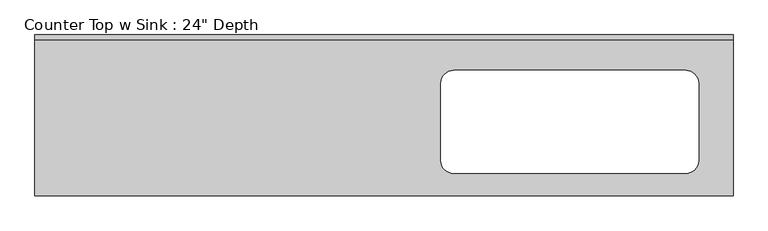
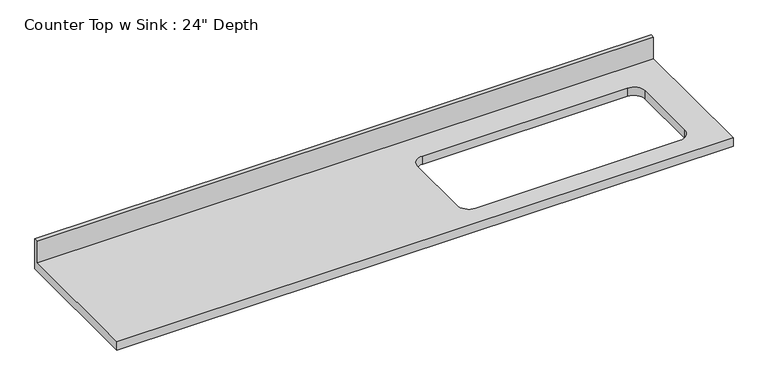
"""IFC4 building model written with IfcOpenShell, lengths in millimetres: furniture geometry."""

from ifc_helpers import new_model, si_unit, frame, origin, place, context, project, spatial, polyline, circle_curve, source, transform, mapped, element, save
from ifc_brep_helpers import plane_surface, revolved_surface, advanced_brep


def furniture_803bf5e8(model_context):
    return source(origin(), model_context, "Body", "AdvancedBrep", [
        advanced_brep(
        [(-1200.4622951, -635.0, 914.4), (1551.9670794, -635.0, 914.4), (1551.9670794, -19.05, 914.4), (-1200.4622951, -19.05, 914.4), (450.5377049, -139.7, 914.4), (1364.9377049, -139.7, 914.4), (1415.7377049, -190.5, 914.4), (1415.7377049, -495.3, 914.4), (1364.9377049, -546.1, 914.4), (450.5377049, -546.1, 914.4), (399.7377049, -495.3, 914.4), (399.7377049, -190.5, 914.4), (1551.9670794, 0.0, 876.3), (1551.9670794, -635.0, 876.3), (-1200.4622951, -635.0, 876.3), (-1200.4622951, 0.0, 876.3), (1364.9377049, -139.7, 876.3), (450.5377049, -139.7, 876.3), (399.7377049, -190.5, 876.3), (399.7377049, -495.3, 876.3), (450.5377049, -546.1, 876.3), (1364.9377049, -546.1, 876.3), (1415.7377049, -495.3, 876.3), (1415.7377049, -190.5, 876.3), (-1200.4622951, 0.0, 1016.0), (1551.9670794, 0.0, 1016.0), (-1200.4622951, -19.05, 1016.0), (1551.9670794, -19.05, 1016.0)],
        [
            (0, 1),
            (1, 2),
            (2, 3),
            (3, 0),
            (4, 5),
            (5, 6, circle_curve(frame((1364.9377049, -190.5, 914.4), z_axis=(0.0, 0.0, -1.0), x_axis=(1.0, 0.0, 0.0)), 50.8)),
            (6, 7),
            (7, 8, circle_curve(frame((1364.9377049, -495.3, 914.4), z_axis=(0.0, 0.0, -1.0), x_axis=(1.0, 0.0, 0.0)), 50.8)),
            (8, 9),
            (9, 10, circle_curve(frame((450.5377049, -495.3, 914.4), z_axis=(0.0, 0.0, -1.0), x_axis=(1.0, 0.0, 0.0)), 50.8)),
            (10, 11),
            (11, 4, circle_curve(frame((450.5377049, -190.5, 914.4), z_axis=(0.0, 0.0, -1.0), x_axis=(1.0, 0.0, 0.0)), 50.8)),
            (12, 13),
            (13, 14),
            (14, 15),
            (15, 12),
            (16, 17),
            (17, 18, circle_curve(frame((450.5377049, -190.5, 876.3), z_axis=(0.0, 0.0, 1.0), x_axis=(1.0, 0.0, 0.0)), 50.8)),
            (18, 19),
            (19, 20, circle_curve(frame((450.5377049, -495.3, 876.3), z_axis=(0.0, 0.0, 1.0), x_axis=(1.0, 0.0, 0.0)), 50.8)),
            (20, 21),
            (21, 22, circle_curve(frame((1364.9377049, -495.3, 876.3), z_axis=(0.0, 0.0, 1.0), x_axis=(1.0, 0.0, 0.0)), 50.8)),
            (22, 23),
            (23, 16, circle_curve(frame((1364.9377049, -190.5, 876.3), z_axis=(0.0, 0.0, 1.0), x_axis=(1.0, 0.0, 0.0)), 50.8)),
            (15, 24),
            (24, 25),
            (25, 12),
            (14, 0),
            (3, 26),
            (26, 24),
            (13, 1),
            (25, 27),
            (27, 2),
            (26, 27),
            (4, 17),
            (16, 5),
            (11, 18),
            (10, 19),
            (9, 20),
            (8, 21),
            (7, 22),
            (6, 23),
        ],
        [
            plane_surface(frame((-1200.4622951, 0.0, 914.4), z_axis=(0.0, 0.0, 1.0), x_axis=(-1.0, 0.0, 0.0))),
            plane_surface(frame((-1200.4622951, 0.0, 876.3), z_axis=(0.0, 0.0, -1.0), x_axis=(1.0, 0.0, 0.0))),
            plane_surface(frame((1551.9670794, 0.0, 914.4), z_axis=(0.0, 1.0, 0.0), x_axis=(0.0, 0.0, -1.0))),
            plane_surface(frame((-1200.4622951, 0.0, 914.4), z_axis=(-1.0, 0.0, 0.0), x_axis=(0.0, 0.0, -1.0))),
            plane_surface(frame((-1200.4622951, -635.0, 914.4), z_axis=(0.0, -1.0, 0.0), x_axis=(0.0, 0.0, -1.0))),
            plane_surface(frame((1551.9670794, -635.0, 914.4), z_axis=(1.0, 0.0, 0.0), x_axis=(0.0, 0.0, -1.0))),
            plane_surface(frame((-1200.4622951, 0.0, 1016.0), z_axis=(0.0, 0.0, 1.0), x_axis=(0.0, -1.0, 0.0))),
            plane_surface(frame((-1200.4622951, -19.05, 1016.0), z_axis=(0.0, -1.0, 0.0), x_axis=(0.0, 0.0, -1.0))),
            plane_surface(frame((1364.9377049, -139.7, 914.4), z_axis=(0.0, -1.0, 0.0), x_axis=(0.0, 0.0, -1.0))),
            revolved_surface(polyline([(501.3377049, -190.5, 914.4), (501.3377049, -190.5, 876.3)]), (450.5377049, -190.5, 876.3), (0.0, 0.0, 1.0)),
            plane_surface(frame((399.7377049, -190.5, 914.4), z_axis=(1.0, 0.0, 0.0), x_axis=(0.0, 0.0, -1.0))),
            revolved_surface(polyline([(501.3377049, -495.3, 914.4), (501.3377049, -495.3, 876.3)]), (450.5377049, -495.3, 876.3), (0.0, 0.0, 1.0)),
            plane_surface(frame((450.5377049, -546.1, 914.4), z_axis=(0.0, 1.0, 0.0), x_axis=(0.0, 0.0, -1.0))),
            revolved_surface(polyline([(1415.7377049, -495.3, 914.4), (1415.7377049, -495.3, 876.3)]), (1364.9377049, -495.3, 876.3), (0.0, 0.0, 1.0)),
            plane_surface(frame((1415.7377049, -495.3, 914.4), z_axis=(-1.0, 0.0, 0.0), x_axis=(0.0, 0.0, -1.0))),
            revolved_surface(polyline([(1415.7377049, -190.5, 914.4), (1415.7377049, -190.5, 876.3)]), (1364.9377049, -190.5, 876.3), (0.0, 0.0, 1.0)),
        ],
        [
            (0, [[1, 2, 3, 4], [5, 6, 7, 8, 9, 10, 11, 12]]),
            (1, [[13, 14, 15, 16], [17, 18, 19, 20, 21, 22, 23, 24]]),
            (2, [[-16, 25, 26, 27]]),
            (3, [[-15, 28, -4, 29, 30, -25]]),
            (4, [[-1, -28, -14, 31]]),
            (5, [[-13, -27, 32, 33, -2, -31]]),
            (6, [[-30, 34, -32, -26]]),
            (7, [[-34, -29, -3, -33]]),
            (8, [[35, -17, 36, -5]]),
            (9, [[-35, -12, 37, -18]]),
            (10, [[-37, -11, 38, -19]]),
            (11, [[-38, -10, 39, -20]]),
            (12, [[-39, -9, 40, -21]]),
            (13, [[-40, -8, 41, -22]]),
            (14, [[-41, -7, 42, -23]]),
            (15, [[-36, -24, -42, -6]]),
        ],
    ),
    ])


if __name__ == "__main__":
    model = new_model("IFC4")
    model_context = context("Model", 3, world=origin())
    ifc_project = project(units=[si_unit("LENGTHUNIT", "METRE", prefix="MILLI")], contexts=[model_context])
    site = spatial("IfcSite", under=ifc_project)
    building = spatial("IfcBuilding", under=site)
    placement = place(None, origin())
    furniture_shape = furniture_803bf5e8(model_context)
    element("IfcFurniture", 1, ObjectType="Counter Top w Sink : 24\" Depth", at=placement, inside=building, context=model_context, shape_type="MappedRepresentation", body=[
        mapped(furniture_shape, transform((0.0, 0.0, 0.0), x_axis=(1.0, 0.0, 0.0), y_axis=(0.0, 1.0, 0.0), z_axis=(0.0, 0.0, 1.0))),
    ])
    save(model, "model.ifc")

# Revit data of these elements
# Type "Counter Top w Sink : 24\" Depth"
#   Assembly Code = "C1030400"
#   Counter Thickness = 0' - 1 1/2"
#   Depth = 2' - 1"
#   Height = 3' - 0"
#   Length [instance default] = 8' - 0"
#   Sink Location [instance default] = 2' - 0"
#   Sink Location To Wall [instance default] = 0' - 6"
#   Sink Opening Depth [instance default] = 1' - 3"
#   Sink Opening Width [instance default] = 3' - 3"
#   Counter Top Material = none
#   Default Elevation = 0
# Element 1 (IfcFurniture, "Counter Top w Sink : 24\" Depth")
#   Length = 9' - 0.36336"
#   Sink Location = 6' - 11"
#   Materials on its faces: "Counter Top"
# Materials
#   "Counter Top": class "Wood", colour RGB 226 177 128, transparency 0
